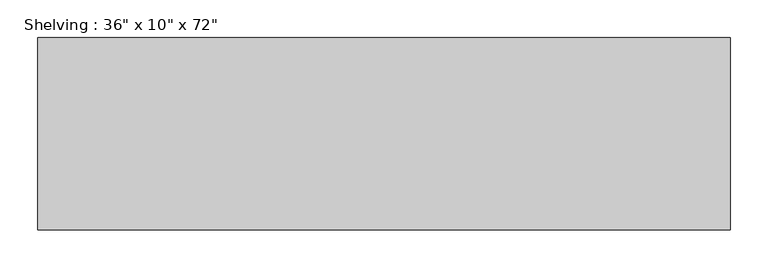
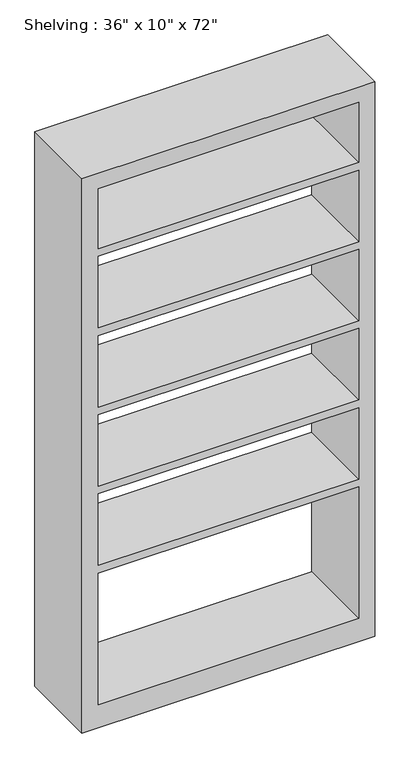
"""IFC4 building model written with IfcOpenShell, lengths in millimetres: furniture geometry."""

from ifc_helpers import new_model, si_unit, frame, origin, place, context, project, spatial, polyline, outline, extrude, source, transform, mapped, element, save


def furniture_417d203a(model_context):
    return source(origin(), model_context, "Body", "SweptSolid", [
        extrude(outline(polyline([(0.0, 457.2), (1828.8, 457.2), (1828.8, -457.2), (0.0, -457.2), (0.0, 457.2)]), holes=[polyline([(1778.0, 406.4), (1580.2428571, 406.4), (1580.2428571, -406.4), (1778.0, -406.4), (1778.0, 406.4)]), polyline([(76.2, 406.4), (76.2, -406.4), (509.8142857, -406.4), (509.8142857, 406.4), (76.2, 406.4)]), polyline([(1057.7285714, -406.4), (1293.5857143, -406.4), (1293.5857143, 406.4), (1057.7285714, 406.4), (1057.7285714, -406.4)]), polyline([(1554.8428571, 406.4), (1318.9857143, 406.4), (1318.9857143, -406.4), (1554.8428571, -406.4), (1554.8428571, 406.4)]), polyline([(1032.3285714, 406.4), (796.4714286, 406.4), (796.4714286, -406.4), (1032.3285714, -406.4), (1032.3285714, 406.4)]), polyline([(771.0714286, 406.4), (535.2142857, 406.4), (535.2142857, -406.4), (771.0714286, -406.4), (771.0714286, 406.4)])]), frame((0.0, -431.8, 0.0), z_axis=(0.0, 1.0, 0.0), x_axis=(0.0, 0.0, 1.0)), (0.0, 0.0, 1.0), 254.0),
    ])


if __name__ == "__main__":
    model = new_model("IFC4")
    model_context = context("Model", 3, world=origin())
    ifc_project = project(units=[si_unit("LENGTHUNIT", "METRE", prefix="MILLI")], contexts=[model_context])
    site = spatial("IfcSite", under=ifc_project)
    building = spatial("IfcBuilding", under=site)
    placement = place(None, origin())
    furniture_shape = furniture_417d203a(model_context)
    element("IfcFurniture", 1, ObjectType="Shelving : 36\" x 10\" x 72\"", at=placement, inside=building, context=model_context, shape_type="MappedRepresentation", body=[
        mapped(furniture_shape, transform((0.0, 0.0, 0.0), x_axis=(1.0, 0.0, 0.0), y_axis=(0.0, 1.0, 0.0), z_axis=(0.0, 0.0, 1.0))),
    ])
    save(model, "model.ifc")

# Revit data of these elements
# Type "Shelving : 36\" x 10\" x 72\""
#   Assembly Code = "E2020200"
#   Depth = 0' - 10"
#   Height = 6' - 0"
#   Width = 3' - 0"
#   Shelving Unit Material = Birch
#   Default Elevation = 0
# Element 1 (IfcFurniture, "Shelving : 36\" x 10\" x 72\"")
#   Materials on its faces: "Birch"
# Materials
#   "Birch": class "Wood", colour RGB 224 178 126, transparency 0, Description = "Betula Alleghaniensis", Cost = 0
